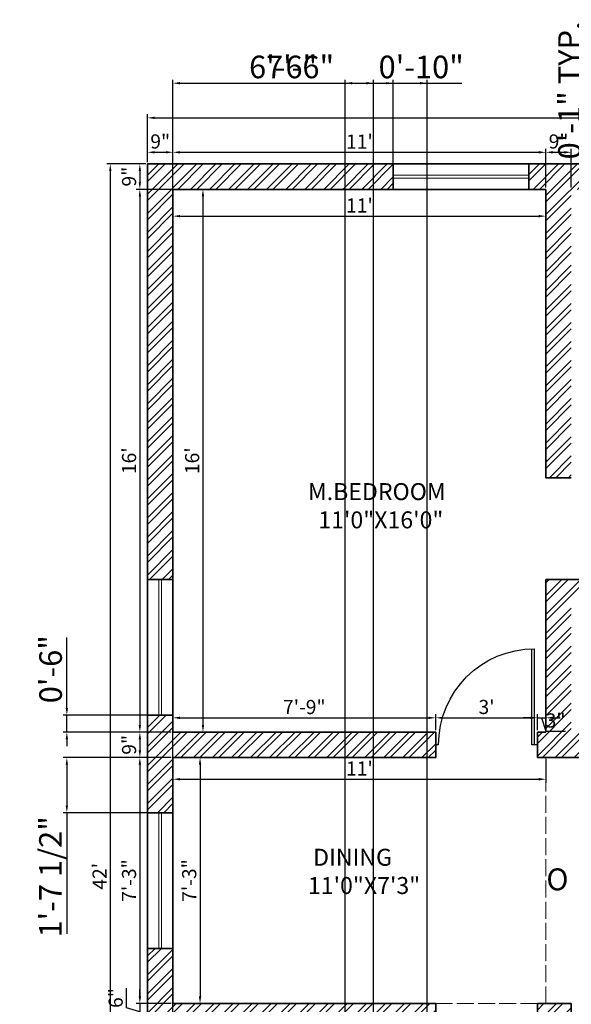
# Model space of a CAD drawing. Units: inches. Extents: x 3595 to 4516, y 2363 to 2965.
# Tile 3 of 12: x 3595 to 3790, y 2606 to 2954. Entities that reach past the tile are written whole.
import ezdxf

# ---------------------------------------------------------------- set-up
doc = ezdxf.new("R2010")
doc.units = ezdxf.units.IN
doc.linetypes.add('ACAD_ISO02W100', pattern=[15, 12, -3])
for name, color, linetype, lineweight in [('A-ANNO-DIMS', 2, 'Continuous', 18), ('A-ANNO-TEXT', 7, 'Continuous', 25), ('A-AREA-IDEN', 7, 'Continuous', 18), ('A-DOOR', 4, 'Continuous', 25), ('A-GLAZ', 4, 'Continuous', 18), ('A-WALL', 7, 'Continuous', 35), ('A-WALL-OVHD', 7, 'ACAD_ISO02W100', 18)]:
    doc.layers.add(name, color=color, linetype=linetype, lineweight=lineweight)
doc.layers.add('A-WALL-PATT', color=251, linetype='Continuous', lineweight=13, true_color=0x636466)
doc.styles.get("Standard").update_dxf_attribs({"font": 'arial.ttf'})
doc.dimstyles.new('ISO-25', dxfattribs={"dimtxt": 8, "dimasz": 2.5, "dimexe": 1.25, "dimexo": 0.625, "dimtad": 1, "dimdec": 1, "dimlunit": 3, "dimtxsty": 'Standard', "dimcen": 2.5, "dimadec": 0, "dimazin": 0, "dimtfac": 1, "dimtdec": 1, "dimtmove": 0, "dimatfit": 3, "dimfxl": 1, "dimarcsym": 0})

# ---------------------------------------------------------------- blocks, each defined once
blk = doc.blocks.new('D1')
for p, q in [((1, 0), (1, 34)), ((2, 0), (2, 33.99)), ((0, 0), (2, 0)), ((35, 0), (36, 0))]:
    blk.add_line(p, q)
at = {"ltscale": 0.5}
blk.add_arc((1, 0), 34, 0, 90, dxfattribs=at)
blk = doc.blocks.new('*D32')
at = {"layer": 'A-ANNO-DIMS', "color": 0, "lineweight": -2, "transparency": 16777216}
for p, q in [((3648.89, 2893.42), (3648.89, 2883.31)), ((3780.89, 2893.42), (3780.89, 2883.31)), ((3651.39, 2884.56), (3778.39, 2884.56))]:
    blk.add_line(p, q, dxfattribs=at)
at = {"layer": 'A-ANNO-DIMS', "color": 0, "transparency": 16777216}
for points in [[(3651.39, 2884.97), (3651.39, 2884.14), (3648.89, 2884.56)], [(3778.39, 2884.97), (3778.39, 2884.14), (3780.89, 2884.56)]]:
    blk.add_solid(points, dxfattribs=at)
at = {"layer": 'Defpoints', "color": 0, "transparency": 16777216}
for p in [(3648.89, 2894.04), (3780.89, 2894.04), (3780.89, 2884.56)]:
    blk.add_point(p, dxfattribs=at)
at = {"layer": 'A-ANNO-DIMS', "color": 0, "transparency": 16777216, "insert": (3714.89, 2887.69), "char_height": 5, "attachment_point": 5}
blk.add_mtext("11'", dxfattribs=at)
blk = doc.blocks.new('*D33')
at = {"layer": 'A-ANNO-DIMS', "color": 0, "lineweight": -2, "transparency": 16777216}
for p, q in [((3649.52, 2894.04), (3660.77, 2894.04)), ((3659.52, 2891.54), (3659.52, 2704.54)), ((3649.52, 2702.04), (3660.77, 2702.04))]:
    blk.add_line(p, q, dxfattribs=at)
at = {"layer": 'A-ANNO-DIMS', "color": 0, "transparency": 16777216}
for points in [[(3659.1, 2891.54), (3659.94, 2891.54), (3659.52, 2894.04)], [(3659.1, 2704.54), (3659.94, 2704.54), (3659.52, 2702.04)]]:
    blk.add_solid(points, dxfattribs=at)
at = {"layer": 'Defpoints', "color": 0, "transparency": 16777216}
for p in [(3648.89, 2894.04), (3648.89, 2702.04), (3659.52, 2702.04)]:
    blk.add_point(p, dxfattribs=at)
at = {"layer": 'A-ANNO-DIMS', "color": 0, "transparency": 16777216, "insert": (3656.34, 2798.04), "char_height": 5, "attachment_point": 5, "rotation": 90}
blk.add_mtext("16'", dxfattribs=at)
blk = doc.blocks.new('*D34')
at = {"layer": 'A-ANNO-DIMS', "color": 0, "lineweight": -2, "transparency": 16777216}
for p, q in [((3648.89, 2702.67), (3648.89, 2708.35)), ((3651.39, 2707.1), (3739.39, 2707.1)), ((3741.89, 2702.67), (3741.89, 2708.35))]:
    blk.add_line(p, q, dxfattribs=at)
at = {"layer": 'A-ANNO-DIMS', "color": 0, "transparency": 16777216}
for points in [[(3651.39, 2707.51), (3651.39, 2706.68), (3648.89, 2707.1)], [(3739.39, 2707.51), (3739.39, 2706.68), (3741.89, 2707.1)]]:
    blk.add_solid(points, dxfattribs=at)
at = {"layer": 'Defpoints', "color": 0, "transparency": 16777216}
for p in [(3741.89, 2707.1), (3648.89, 2702.04), (3741.89, 2702.04)]:
    blk.add_point(p, dxfattribs=at)
at = {"layer": 'A-ANNO-DIMS', "color": 0, "transparency": 16777216, "insert": (3695.39, 2710.27), "char_height": 5, "attachment_point": 5}
blk.add_mtext('7\'-9"', dxfattribs=at)
blk = doc.blocks.new('*D35')
at = {"layer": 'A-ANNO-DIMS', "color": 0, "lineweight": -2, "transparency": 16777216}
for p, q in [((3741.89, 2702.67), (3741.89, 2708.35)), ((3744.39, 2707.1), (3775.39, 2707.1)), ((3777.89, 2702.67), (3777.89, 2708.35))]:
    blk.add_line(p, q, dxfattribs=at)
at = {"layer": 'A-ANNO-DIMS', "color": 0, "transparency": 16777216}
for points in [[(3744.39, 2707.51), (3744.39, 2706.68), (3741.89, 2707.1)], [(3775.39, 2707.51), (3775.39, 2706.68), (3777.89, 2707.1)]]:
    blk.add_solid(points, dxfattribs=at)
at = {"layer": 'Defpoints', "color": 0, "transparency": 16777216}
for p in [(3777.89, 2707.1), (3741.89, 2702.04), (3777.89, 2702.04)]:
    blk.add_point(p, dxfattribs=at)
at = {"layer": 'A-ANNO-DIMS', "color": 0, "transparency": 16777216, "insert": (3759.89, 2710.28), "char_height": 5, "attachment_point": 5}
blk.add_mtext("3'", dxfattribs=at)
blk = doc.blocks.new('*D36')
at = {"layer": 'A-ANNO-DIMS', "color": 0, "lineweight": -2, "transparency": 16777216}
for p, q in [((3775.39, 2707.1), (3772.89, 2707.1)), ((3777.89, 2702.67), (3777.89, 2708.35)), ((3777.89, 2707.1), (3780.89, 2707.1)), ((3777.89, 2707.1), (3780.89, 2707.1)), ((3779.39, 2707.1), (3780.82, 2702.35)), ((3780.89, 2706.47), (3780.89, 2705.85)), ((3783.39, 2707.1), (3785.89, 2707.1)), ((3780.82, 2702.35), (3787.81, 2702.35))]:
    blk.add_line(p, q, dxfattribs=at)
at = {"layer": 'A-ANNO-DIMS', "color": 0, "transparency": 16777216}
for points in [[(3775.39, 2707.51), (3775.39, 2706.68), (3777.89, 2707.1)], [(3783.39, 2707.51), (3783.39, 2706.68), (3780.89, 2707.1)]]:
    blk.add_solid(points, dxfattribs=at)
at = {"layer": 'Defpoints', "color": 0, "transparency": 16777216}
for p in [(3780.89, 2707.1), (3780.89, 2707.1), (3777.89, 2702.04)]:
    blk.add_point(p, dxfattribs=at)
at = {"layer": 'A-ANNO-DIMS', "color": 0, "transparency": 16777216, "insert": (3784.31, 2705.53), "char_height": 5, "attachment_point": 5}
blk.add_mtext('3"', dxfattribs=at)
blk = doc.blocks.new('*D46')
at = {"layer": 'A-ANNO-DIMS', "color": 0, "lineweight": -2, "transparency": 16777216}
for p, q in [((3649.52, 2693.04), (3659.74, 2693.04)), ((3658.49, 2690.54), (3658.49, 2608.54)), ((3649.52, 2606.04), (3659.74, 2606.04))]:
    blk.add_line(p, q, dxfattribs=at)
at = {"layer": 'A-ANNO-DIMS', "color": 0, "transparency": 16777216}
for points in [[(3658.07, 2690.54), (3658.91, 2690.54), (3658.49, 2693.04)], [(3658.07, 2608.54), (3658.91, 2608.54), (3658.49, 2606.04)]]:
    blk.add_solid(points, dxfattribs=at)
at = {"layer": 'Defpoints', "color": 0, "transparency": 16777216}
for p in [(3648.89, 2693.04), (3648.89, 2606.04), (3658.49, 2606.04)]:
    blk.add_point(p, dxfattribs=at)
at = {"layer": 'A-ANNO-DIMS', "color": 0, "transparency": 16777216, "insert": (3655.31, 2649.54), "char_height": 5, "attachment_point": 5, "rotation": 90}
blk.add_mtext('7\'-3"', dxfattribs=at)
blk = doc.blocks.new('*D47')
at = {"layer": 'A-ANNO-DIMS', "color": 0, "lineweight": -2, "transparency": 16777216}
for p, q in [((3648.89, 2692.42), (3648.89, 2684.12)), ((3780.89, 2692.42), (3780.89, 2684.12)), ((3651.39, 2685.37), (3778.39, 2685.37))]:
    blk.add_line(p, q, dxfattribs=at)
at = {"layer": 'A-ANNO-DIMS', "color": 0, "transparency": 16777216}
for points in [[(3651.39, 2685.79), (3651.39, 2684.95), (3648.89, 2685.37)], [(3778.39, 2685.79), (3778.39, 2684.95), (3780.89, 2685.37)]]:
    blk.add_solid(points, dxfattribs=at)
at = {"layer": 'Defpoints', "color": 0, "transparency": 16777216}
for p in [(3648.89, 2693.04), (3780.89, 2693.04), (3780.89, 2685.37)]:
    blk.add_point(p, dxfattribs=at)
at = {"layer": 'A-ANNO-DIMS', "color": 0, "transparency": 16777216, "insert": (3714.89, 2688.5), "char_height": 5, "attachment_point": 5}
blk.add_mtext("11'", dxfattribs=at)
blk = doc.blocks.new('*D51')
at = {"layer": 'A-ANNO-DIMS', "color": 0, "lineweight": -2, "transparency": 16777216}
for p, q in [((3790.52, 2693.04), (3802.44, 2693.04)), ((3801.19, 2488.54), (3801.19, 2690.54)), ((3790.52, 2486.04), (3802.44, 2486.04))]:
    blk.add_line(p, q, dxfattribs=at)
at = {"layer": 'A-ANNO-DIMS', "color": 0, "transparency": 16777216}
for points in [[(3800.78, 2690.54), (3801.61, 2690.54), (3801.19, 2693.04)], [(3800.78, 2488.54), (3801.61, 2488.54), (3801.19, 2486.04)]]:
    blk.add_solid(points, dxfattribs=at)
at = {"layer": 'Defpoints', "color": 0, "transparency": 16777216}
for p in [(3789.89, 2693.04), (3801.19, 2693.04), (3789.89, 2486.04)]:
    blk.add_point(p, dxfattribs=at)
at = {"layer": 'A-ANNO-DIMS', "color": 0, "transparency": 16777216, "insert": (3798.01, 2589.54), "char_height": 5, "attachment_point": 5, "rotation": 90}
blk.add_mtext('17\'-3"', dxfattribs=at)
blk = doc.blocks.new('*D60')
at = {"layer": 'A-ANNO-DIMS', "color": 0, "lineweight": -2, "transparency": 16777216}
for p, q in [((3639.89, 2903.67), (3639.89, 2908.4)), ((3648.89, 2894.67), (3648.89, 2908.4)), ((3642.39, 2907.15), (3646.39, 2907.15))]:
    blk.add_line(p, q, dxfattribs=at)
at = {"layer": 'A-ANNO-DIMS', "color": 0, "transparency": 16777216}
for points in [[(3642.39, 2907.57), (3642.39, 2906.73), (3639.89, 2907.15)], [(3646.39, 2907.57), (3646.39, 2906.73), (3648.89, 2907.15)]]:
    blk.add_solid(points, dxfattribs=at)
at = {"layer": 'Defpoints', "color": 0, "transparency": 16777216}
for p in [(3648.89, 2907.15), (3639.89, 2903.04), (3648.89, 2894.04)]:
    blk.add_point(p, dxfattribs=at)
at = {"layer": 'A-ANNO-DIMS', "color": 0, "transparency": 16777216, "insert": (3644.39, 2910.33), "char_height": 5, "attachment_point": 5}
blk.add_mtext('9"', dxfattribs=at)
blk = doc.blocks.new('*D61')
at = {"layer": 'A-ANNO-DIMS', "color": 0, "lineweight": -2, "transparency": 16777216}
for p, q in [((3648.89, 2894.67), (3648.89, 2908.4)), ((3780.89, 2894.67), (3780.89, 2908.4)), ((3651.39, 2907.15), (3778.39, 2907.15))]:
    blk.add_line(p, q, dxfattribs=at)
at = {"layer": 'A-ANNO-DIMS', "color": 0, "transparency": 16777216}
for points in [[(3651.39, 2907.57), (3651.39, 2906.73), (3648.89, 2907.15)], [(3778.39, 2907.57), (3778.39, 2906.73), (3780.89, 2907.15)]]:
    blk.add_solid(points, dxfattribs=at)
at = {"layer": 'Defpoints', "color": 0, "transparency": 16777216}
for p in [(3780.89, 2907.15), (3648.89, 2894.04), (3780.89, 2894.04)]:
    blk.add_point(p, dxfattribs=at)
at = {"layer": 'A-ANNO-DIMS', "color": 0, "transparency": 16777216, "insert": (3714.89, 2910.29), "char_height": 5, "attachment_point": 5}
blk.add_mtext("11'", dxfattribs=at)
blk = doc.blocks.new('*D62')
at = {"layer": 'A-ANNO-DIMS', "color": 0, "lineweight": -2, "transparency": 16777216}
for p, q in [((3780.89, 2894.67), (3780.89, 2908.4)), ((3789.89, 2894.67), (3789.89, 2908.4)), ((3783.39, 2907.15), (3787.39, 2907.15))]:
    blk.add_line(p, q, dxfattribs=at)
at = {"layer": 'A-ANNO-DIMS', "color": 0, "transparency": 16777216}
for points in [[(3783.39, 2907.57), (3783.39, 2906.73), (3780.89, 2907.15)], [(3787.39, 2907.57), (3787.39, 2906.73), (3789.89, 2907.15)]]:
    blk.add_solid(points, dxfattribs=at)
at = {"layer": 'Defpoints', "color": 0, "transparency": 16777216}
for p in [(3789.89, 2907.15), (3780.89, 2894.04), (3789.89, 2894.04)]:
    blk.add_point(p, dxfattribs=at)
at = {"layer": 'A-ANNO-DIMS', "color": 0, "transparency": 16777216, "insert": (3785.39, 2910.33), "char_height": 5, "attachment_point": 5}
blk.add_mtext('9"', dxfattribs=at)
blk = doc.blocks.new('*D69')
at = {"layer": 'A-ANNO-DIMS', "color": 0, "lineweight": -2, "transparency": 16777216}
for p, q in [((3639.27, 2903.04), (3635.93, 2903.04)), ((3637.18, 2900.54), (3637.18, 2896.54)), ((3648.27, 2894.04), (3635.93, 2894.04))]:
    blk.add_line(p, q, dxfattribs=at)
at = {"layer": 'A-ANNO-DIMS', "color": 0, "transparency": 16777216}
for points in [[(3636.77, 2900.54), (3637.6, 2900.54), (3637.18, 2903.04)], [(3636.77, 2896.54), (3637.6, 2896.54), (3637.18, 2894.04)]]:
    blk.add_solid(points, dxfattribs=at)
at = {"layer": 'Defpoints', "color": 0, "transparency": 16777216}
for p in [(3639.89, 2903.04), (3637.18, 2894.04), (3648.89, 2894.04)]:
    blk.add_point(p, dxfattribs=at)
at = {"layer": 'A-ANNO-DIMS', "color": 0, "transparency": 16777216, "insert": (3634.01, 2898.54), "char_height": 5, "attachment_point": 5, "rotation": 90}
blk.add_mtext('9"', dxfattribs=at)
blk = doc.blocks.new('*D70')
at = {"layer": 'A-ANNO-DIMS', "color": 0, "lineweight": -2, "transparency": 16777216}
for p, q in [((3648.27, 2894.04), (3635.93, 2894.04)), ((3637.18, 2891.54), (3637.18, 2704.54)), ((3648.27, 2702.04), (3635.93, 2702.04))]:
    blk.add_line(p, q, dxfattribs=at)
at = {"layer": 'A-ANNO-DIMS', "color": 0, "transparency": 16777216}
for points in [[(3636.77, 2891.54), (3637.6, 2891.54), (3637.18, 2894.04)], [(3636.77, 2704.54), (3637.6, 2704.54), (3637.18, 2702.04)]]:
    blk.add_solid(points, dxfattribs=at)
at = {"layer": 'Defpoints', "color": 0, "transparency": 16777216}
for p in [(3648.89, 2894.04), (3637.18, 2702.04), (3648.89, 2702.04)]:
    blk.add_point(p, dxfattribs=at)
at = {"layer": 'A-ANNO-DIMS', "color": 0, "transparency": 16777216, "insert": (3634.01, 2798.04), "char_height": 5, "attachment_point": 5, "rotation": 90}
blk.add_mtext("16'", dxfattribs=at)
blk = doc.blocks.new('*D71')
at = {"layer": 'A-ANNO-DIMS', "color": 0, "lineweight": -2, "transparency": 16777216}
for p, q in [((3648.27, 2702.04), (3635.93, 2702.04)), ((3637.18, 2699.54), (3637.18, 2695.54)), ((3648.27, 2693.04), (3635.93, 2693.04))]:
    blk.add_line(p, q, dxfattribs=at)
at = {"layer": 'A-ANNO-DIMS', "color": 0, "transparency": 16777216}
for points in [[(3636.77, 2699.54), (3637.6, 2699.54), (3637.18, 2702.04)], [(3636.77, 2695.54), (3637.6, 2695.54), (3637.18, 2693.04)]]:
    blk.add_solid(points, dxfattribs=at)
at = {"layer": 'Defpoints', "color": 0, "transparency": 16777216}
for p in [(3648.89, 2702.04), (3637.18, 2693.04), (3648.89, 2693.04)]:
    blk.add_point(p, dxfattribs=at)
at = {"layer": 'A-ANNO-DIMS', "color": 0, "transparency": 16777216, "insert": (3634.01, 2697.54), "char_height": 5, "attachment_point": 5, "rotation": 90}
blk.add_mtext('9"', dxfattribs=at)
blk = doc.blocks.new('*D72')
at = {"layer": 'A-ANNO-DIMS', "color": 0, "lineweight": -2, "transparency": 16777216}
for p, q in [((3648.27, 2693.04), (3635.93, 2693.04)), ((3637.18, 2690.54), (3637.18, 2608.54)), ((3648.27, 2606.04), (3635.93, 2606.04))]:
    blk.add_line(p, q, dxfattribs=at)
at = {"layer": 'A-ANNO-DIMS', "color": 0, "transparency": 16777216}
for points in [[(3636.77, 2690.54), (3637.6, 2690.54), (3637.18, 2693.04)], [(3636.77, 2608.54), (3637.6, 2608.54), (3637.18, 2606.04)]]:
    blk.add_solid(points, dxfattribs=at)
at = {"layer": 'Defpoints', "color": 0, "transparency": 16777216}
for p in [(3648.89, 2693.04), (3637.18, 2606.04), (3648.89, 2606.04)]:
    blk.add_point(p, dxfattribs=at)
at = {"layer": 'A-ANNO-DIMS', "color": 0, "transparency": 16777216, "insert": (3634, 2649.54), "char_height": 5, "attachment_point": 5, "rotation": 90}
blk.add_mtext('7\'-3"', dxfattribs=at)
blk = doc.blocks.new('*D73')
at = {"layer": 'A-ANNO-DIMS', "color": 0, "lineweight": -2, "transparency": 16777216}
for p, q in [((3632.44, 2604.47), (3632.44, 2611.49)), ((3637.18, 2608.54), (3637.18, 2611.04)), ((3648.27, 2606.04), (3635.93, 2606.04)), ((3637.18, 2606.04), (3637.18, 2600.04)), ((3637.18, 2606.04), (3637.18, 2600.04)), ((3637.18, 2603.04), (3632.44, 2604.47)), ((3648.27, 2600.04), (3635.93, 2600.04)), ((3637.18, 2597.54), (3637.18, 2595.04))]:
    blk.add_line(p, q, dxfattribs=at)
at = {"layer": 'A-ANNO-DIMS', "color": 0, "transparency": 16777216}
for points in [[(3636.77, 2608.54), (3637.6, 2608.54), (3637.18, 2606.04)], [(3636.77, 2597.54), (3637.6, 2597.54), (3637.18, 2600.04)]]:
    blk.add_solid(points, dxfattribs=at)
at = {"layer": 'Defpoints', "color": 0, "transparency": 16777216}
for p in [(3648.89, 2606.04), (3637.18, 2600.04), (3648.89, 2600.04)]:
    blk.add_point(p, dxfattribs=at)
at = {"layer": 'A-ANNO-DIMS', "color": 0, "transparency": 16777216, "insert": (3629.27, 2607.98), "char_height": 5, "attachment_point": 5, "rotation": 90}
blk.add_mtext('6"', dxfattribs=at)
blk = doc.blocks.new('*D89')
at = {"layer": 'A-ANNO-DIMS', "color": 0, "lineweight": -2, "transparency": 16777216}
for p, q in [((3639.89, 2903.67), (3639.89, 2920.58)), ((3642.39, 2919.33), (3997.39, 2919.33)), ((3999.89, 2903.67), (3999.89, 2920.58))]:
    blk.add_line(p, q, dxfattribs=at)
at = {"layer": 'A-ANNO-DIMS', "color": 0, "transparency": 16777216}
for points in [[(3642.39, 2919.75), (3642.39, 2918.91), (3639.89, 2919.33)], [(3997.39, 2919.75), (3997.39, 2918.91), (3999.89, 2919.33)]]:
    blk.add_solid(points, dxfattribs=at)
at = {"layer": 'Defpoints', "color": 0, "transparency": 16777216}
for p in [(3999.89, 2919.33), (3639.89, 2903.04), (3999.89, 2903.04)]:
    blk.add_point(p, dxfattribs=at)
at = {"layer": 'A-ANNO-DIMS', "color": 0, "transparency": 16777216, "insert": (3819.89, 2922.51), "char_height": 5, "attachment_point": 5}
blk.add_mtext("30'", dxfattribs=at)
blk = doc.blocks.new('*D90')
at = {"layer": 'A-ANNO-DIMS', "color": 0, "lineweight": -2, "transparency": 16777216}
for p, q in [((3639.27, 2903.04), (3625.46, 2903.04)), ((3626.71, 2900.54), (3626.71, 2401.54)), ((3639.27, 2399.04), (3625.46, 2399.04))]:
    blk.add_line(p, q, dxfattribs=at)
at = {"layer": 'A-ANNO-DIMS', "color": 0, "transparency": 16777216}
for points in [[(3626.3, 2900.54), (3627.13, 2900.54), (3626.71, 2903.04)], [(3626.3, 2401.54), (3627.13, 2401.54), (3626.71, 2399.04)]]:
    blk.add_solid(points, dxfattribs=at)
at = {"layer": 'Defpoints', "color": 0, "transparency": 16777216}
for p in [(3639.89, 2903.04), (3626.71, 2399.04), (3639.89, 2399.04)]:
    blk.add_point(p, dxfattribs=at)
at = {"layer": 'A-ANNO-DIMS', "color": 0, "transparency": 16777216, "insert": (3623.58, 2651.04), "char_height": 5, "attachment_point": 5, "rotation": 90}
blk.add_mtext("42'", dxfattribs=at)
blk = doc.blocks.new('WIN-GLAZING-48IN')
for p, q in [((0, 1), (48, 1)), ((0, 0), (48, 0))]:
    blk.add_line(p, q)
blk = doc.blocks.new('*D108')
at = {"layer": 'A-ANNO-DIMS', "color": 0, "lineweight": -2, "transparency": 16777216}
for p, q in [((3794.99, 2901.54), (3794.99, 2954.06)), ((3799.77, 2899.04), (3793.74, 2899.04)), ((3799.77, 2898.04), (3793.74, 2898.04)), ((3794.99, 2898.04), (3794.99, 2899.04)), ((3794.99, 2895.54), (3794.99, 2893.04))]:
    blk.add_line(p, q, dxfattribs=at)
at = {"layer": 'A-ANNO-DIMS', "color": 0, "transparency": 16777216}
for points in [[(3794.58, 2901.54), (3795.41, 2901.54), (3794.99, 2899.04)], [(3794.58, 2895.54), (3795.41, 2895.54), (3794.99, 2898.04)]]:
    blk.add_solid(points, dxfattribs=at)
at = {"layer": 'Defpoints', "color": 0, "transparency": 16777216}
for p in [(3794.99, 2899.04), (3800.39, 2899.04), (3800.39, 2898.04)]:
    blk.add_point(p, dxfattribs=at)
at = {"layer": 'A-ANNO-DIMS', "color": 0, "transparency": 16777216, "insert": (3790.28, 2929.05), "char_height": 8, "attachment_point": 5, "rotation": 90}
blk.add_mtext('0\'-1" TYP.', dxfattribs=at)
blk = doc.blocks.new('*D147')
at = {"layer": 'A-ANNO-DIMS', "color": 0, "lineweight": -2, "transparency": 16777216}
for p, q in [((3648.89, 2894.67), (3648.89, 2932.84)), ((3726.89, 2894.67), (3726.89, 2932.84)), ((3651.39, 2931.59), (3724.39, 2931.59))]:
    blk.add_line(p, q, dxfattribs=at)
at = {"layer": 'A-ANNO-DIMS', "color": 0, "transparency": 16777216}
for points in [[(3651.39, 2932.01), (3651.39, 2931.18), (3648.89, 2931.59)], [(3724.39, 2932.01), (3724.39, 2931.18), (3726.89, 2931.59)]]:
    blk.add_solid(points, dxfattribs=at)
at = {"layer": 'Defpoints', "color": 0, "transparency": 16777216}
for p in [(3726.89, 2931.59), (3648.89, 2894.04), (3726.89, 2894.04)]:
    blk.add_point(p, dxfattribs=at)
at = {"layer": 'A-ANNO-DIMS', "color": 0, "transparency": 16777216, "insert": (3687.89, 2936.3), "char_height": 8, "attachment_point": 5}
blk.add_mtext('6\'-6"', dxfattribs=at)
blk = doc.blocks.new('*D150')
at = {"layer": 'A-ANNO-DIMS', "color": 0, "lineweight": -2, "transparency": 16777216}
for p, q in [((3611.34, 2710.54), (3611.34, 2735.56)), ((3648.27, 2708.04), (3610.09, 2708.04)), ((3611.34, 2702.04), (3611.34, 2708.04)), ((3648.27, 2702.04), (3610.09, 2702.04)), ((3611.34, 2699.54), (3611.34, 2697.04))]:
    blk.add_line(p, q, dxfattribs=at)
at = {"layer": 'A-ANNO-DIMS', "color": 0, "transparency": 16777216}
for points in [[(3610.93, 2710.54), (3611.76, 2710.54), (3611.34, 2708.04)], [(3610.93, 2699.54), (3611.76, 2699.54), (3611.34, 2702.04)]]:
    blk.add_solid(points, dxfattribs=at)
at = {"layer": 'Defpoints', "color": 0, "transparency": 16777216}
for p in [(3611.34, 2708.04), (3648.89, 2708.04), (3648.89, 2702.04)]:
    blk.add_point(p, dxfattribs=at)
at = {"layer": 'A-ANNO-DIMS', "color": 0, "transparency": 16777216, "insert": (3606.63, 2724.3), "char_height": 8, "attachment_point": 5, "rotation": 90}
blk.add_mtext('0\'-6"', dxfattribs=at)
blk = doc.blocks.new('*D151')
at = {"layer": 'A-ANNO-DIMS', "color": 0, "lineweight": -2, "transparency": 16777216}
for p, q in [((3648.27, 2693.04), (3610.09, 2693.04)), ((3611.34, 2690.54), (3611.34, 2676.04)), ((3648.27, 2673.54), (3610.09, 2673.54)), ((3611.34, 2673.54), (3611.34, 2630.64))]:
    blk.add_line(p, q, dxfattribs=at)
at = {"layer": 'A-ANNO-DIMS', "color": 0, "transparency": 16777216}
for points in [[(3610.93, 2690.54), (3611.76, 2690.54), (3611.34, 2693.04)], [(3610.93, 2676.04), (3611.76, 2676.04), (3611.34, 2673.54)]]:
    blk.add_solid(points, dxfattribs=at)
at = {"layer": 'Defpoints', "color": 0, "transparency": 16777216}
for p in [(3648.89, 2693.04), (3611.34, 2673.54), (3648.89, 2673.54)]:
    blk.add_point(p, dxfattribs=at)
at = {"layer": 'A-ANNO-DIMS', "color": 0, "transparency": 16777216, "insert": (3606.58, 2650.84), "char_height": 8, "attachment_point": 5, "rotation": 90}
blk.add_mtext('1\'-7 1/2"', dxfattribs=at)
blk = doc.blocks.new('*D156')
at = {"layer": 'A-ANNO-DIMS', "color": 0, "lineweight": -2, "transparency": 16777216}
for p, q in [((3648.89, 2486.67), (3648.89, 2932.84)), ((3738.89, 2486.67), (3738.89, 2932.84)), ((3651.39, 2931.59), (3736.39, 2931.59))]:
    blk.add_line(p, q, dxfattribs=at)
at = {"layer": 'A-ANNO-DIMS', "color": 0, "transparency": 16777216}
for points in [[(3651.39, 2932.01), (3651.39, 2931.18), (3648.89, 2931.59)], [(3736.39, 2932.01), (3736.39, 2931.18), (3738.89, 2931.59)]]:
    blk.add_solid(points, dxfattribs=at)
at = {"layer": 'Defpoints', "color": 0, "transparency": 16777216}
for p in [(3738.89, 2931.59), (3648.89, 2486.04), (3738.89, 2486.04)]:
    blk.add_point(p, dxfattribs=at)
at = {"layer": 'A-ANNO-DIMS', "color": 0, "transparency": 16777216, "insert": (3693.89, 2936.3), "char_height": 8, "attachment_point": 5}
blk.add_mtext('7\'-6"', dxfattribs=at)
blk = doc.blocks.new('*D159')
at = {"layer": 'A-ANNO-DIMS', "color": 0, "lineweight": -2, "transparency": 16777216}
for p, q in [((3709.89, 2405.67), (3709.89, 2932.84)), ((3719.89, 2405.67), (3719.89, 2932.84)), ((3712.39, 2931.59), (3717.39, 2931.59)), ((3719.89, 2931.59), (3751.12, 2931.59))]:
    blk.add_line(p, q, dxfattribs=at)
at = {"layer": 'A-ANNO-DIMS', "color": 0, "transparency": 16777216}
for points in [[(3712.39, 2932.01), (3712.39, 2931.18), (3709.89, 2931.59)], [(3717.39, 2932.01), (3717.39, 2931.18), (3719.89, 2931.59)]]:
    blk.add_solid(points, dxfattribs=at)
at = {"layer": 'Defpoints', "color": 0, "transparency": 16777216}
for p in [(3719.89, 2931.59), (3709.89, 2405.04), (3719.89, 2405.04)]:
    blk.add_point(p, dxfattribs=at)
at = {"layer": 'A-ANNO-DIMS', "color": 0, "transparency": 16777216, "insert": (3736.76, 2936.3), "char_height": 8, "attachment_point": 5}
blk.add_mtext('0\'-10"', dxfattribs=at)

msp = doc.modelspace()

# ---------------------------------------------------------------- hatches: boundary and pattern name
at = {"layer": 'A-WALL-PATT'}
h = msp.add_hatch(dxfattribs=at)
h.set_pattern_fill('ANSI32', color=256, scale=0.5)
h.paths.add_polyline_path([(3648.89, 2894.04), (3726.89, 2894.04), (3726.89, 2903.04), (3639.89, 2903.04), (3639.89, 2756.04), (3648.89, 2756.04)])
h.paths.add_polyline_path([(3800.39, 2903.04), (3774.89, 2903.04), (3774.89, 2894.04), (3780.89, 2894.04), (3780.89, 2792.04), (3789.89, 2792.04), (3789.89, 2894.04), (3800.39, 2894.04)])
h.paths.add_polyline_path([(3882.89, 2903.04), (3836.39, 2903.04), (3836.39, 2894.04), (3846.89, 2894.04), (3846.89, 2798.04), (3819.89, 2798.04), (3819.89, 2792.04), (3846.89, 2792.04), (3846.89, 2756.04), (3780.89, 2756.04), (3780.89, 2702.04), (3777.89, 2702.04), (3777.89, 2693.04), (3800.39, 2693.04), (3800.39, 2702.04), (3789.89, 2702.04), (3789.89, 2750.04), (3846.89, 2750.04), (3846.89, 2702.04), (3836.39, 2702.04), (3836.39, 2693.04), (3951.89, 2693.04), (3951.89, 2702.04), (3852.89, 2702.04), (3852.89, 2840.04), (3954.89, 2840.04), (3954.89, 2846.04), (3852.89, 2846.04), (3852.89, 2894.04), (3882.89, 2894.04)])
h.paths.add_polyline_path([(3999.89, 2903.04), (3918.89, 2903.04), (3918.89, 2894.04), (3948.89, 2894.04), (3948.89, 2876.04), (3954.89, 2876.04), (3954.89, 2894.04), (3990.89, 2894.04), (3990.89, 2795.04), (3999.89, 2795.04)])
h.paths.add_polyline_path([(3741.89, 2702.04), (3648.89, 2702.04), (3648.89, 2708.04), (3639.89, 2708.04), (3639.89, 2673.54), (3648.89, 2673.54), (3648.89, 2693.04), (3741.89, 2693.04)])
h.paths.add_polyline_path([(3648.89, 2600.04), (3741.89, 2600.04), (3741.89, 2606.04), (3648.89, 2606.04), (3648.89, 2625.54), (3639.89, 2625.54), (3639.89, 2561.04), (3648.89, 2561.04)])
h.paths.add_polyline_path([(3648.89, 2525.04), (3639.89, 2525.04), (3639.89, 2399.04), (3789.89, 2399.04), (3789.89, 2405.04), (3648.89, 2405.04), (3648.89, 2477.04), (3738.89, 2477.04), (3738.89, 2486.04), (3648.89, 2486.04)])
h.paths.add_polyline_path([(3789.89, 2606.04), (3777.89, 2606.04), (3777.89, 2600.04), (3780.89, 2600.04), (3780.89, 2486.04), (3774.89, 2486.04), (3774.89, 2477.04), (3831.89, 2477.04), (3831.89, 2486.04), (3789.89, 2486.04)])
h.paths.add_polyline_path([(3939.89, 2486.04), (3897.89, 2486.04), (3897.89, 2477.04), (3939.89, 2477.04)])
h.paths.add_polyline_path([(3999.89, 2511.54), (3990.89, 2511.54), (3990.89, 2486.04), (3987.89, 2486.04), (3987.89, 2477.04), (3999.89, 2477.04)])
h.paths.add_polyline_path([(3999.89, 2607.54), (3990.89, 2607.54), (3990.89, 2571.54), (3999.89, 2571.54)])
h.paths.add_polyline_path([(3999.89, 2747.04), (3990.89, 2747.04), (3990.89, 2702.04), (3987.89, 2702.04), (3987.89, 2693.04), (3990.89, 2693.04), (3990.89, 2667.54), (3999.89, 2667.54)])

# ---------------------------------------------------------------- linework, layer by layer
at = {"layer": 'A-WALL'}
for p, q in [((3726.89, 2894.04), (3726.89, 2903.04)), ((3774.89, 2894.04), (3774.89, 2903.04)), ((3648.89, 2894.04), (3780.89, 2894.04)), ((3648.89, 2702.04), (3648.89, 2894.04)), ((3780.89, 2792.04), (3780.89, 2894.04)), ((3780.89, 2792.04), (3789.89, 2792.04)), ((3639.89, 2756.04), (3648.89, 2756.04)), ((3780.89, 2756.04), (3846.89, 2756.04)), ((3780.89, 2702.04), (3780.89, 2756.04)), ((3639.89, 2708.04), (3648.89, 2708.04)), ((3648.89, 2702.04), (3741.89, 2702.04)), ((3741.89, 2693.04), (3741.89, 2702.04)), ((3777.89, 2693.04), (3777.89, 2702.04)), ((3777.89, 2702.04), (3780.89, 2702.04)), ((3648.89, 2693.04), (3741.89, 2693.04)), ((3648.89, 2606.04), (3648.89, 2693.04)), ((3777.89, 2693.04), (3800.39, 2693.04)), ((3639.89, 2673.54), (3648.89, 2673.54)), ((3639.89, 2625.54), (3648.89, 2625.54)), ((3648.89, 2606.04), (3741.89, 2606.04)), ((3741.89, 2606.04), (3741.89, 2600.04)), ((3777.89, 2606.04), (3777.89, 2600.04)), ((3777.89, 2606.04), (3789.89, 2606.04)), ((3789.89, 2486.04), (3789.89, 2606.04))]:
    msp.add_line(p, q, dxfattribs=at)
msp.add_lwpolyline([(3789.89, 2399.04), (3639.89, 2399.04), (3639.89, 2903.04), (3999.89, 2903.04), (3999.89, 2477.04)], dxfattribs=at)
at = {"layer": 'A-WALL-OVHD', "ltscale": 0.5}
for p, q in [((3780.89, 2606.04), (3780.89, 2693.04)), ((3741.89, 2606.04), (3777.89, 2606.04))]:
    msp.add_line(p, q, dxfattribs=at)

# ---------------------------------------------------------------- block references
at = {"layer": 'A-DOOR', "xscale": -1}
msp.add_blockref('D1', (3777.89, 2697.54), dxfattribs=at)
at = {"layer": 'A-GLAZ'}
msp.add_blockref('WIN-GLAZING-48IN', (3726.89, 2898.04), dxfattribs=at)
at = {"layer": 'A-GLAZ', "rotation": 269.9999999999989}
for p in [(3643.89, 2756.04), (3643.89, 2673.54)]:
    msp.add_blockref('WIN-GLAZING-48IN', p, dxfattribs=at)

# ---------------------------------------------------------------- texts
at = {"layer": 'A-ANNO-TEXT'}
msp.add_text('O', height=7.75, dxfattribs=at).set_placement((3781.06, 2646.07))
at = {"layer": 'A-AREA-IDEN', "char_height": 6, "attachment_point": 1}
for s, insert in [('{\\fTimes New Roman|b0|i0|c0|p18;M.BEDROOM\\P  11\'0"X16\'0"}', (3696.68, 2790.12)), ('{\\fTimes New Roman|b0|i0|c0|p18; DINING\\P11\'0"X7\'3"}', (3696.68, 2660.77))]:
    msp.add_mtext_dynamic_manual_height_columns(s, width=67.3508, gutter_width=12.5, heights=[0], dxfattribs=dict(at, insert=insert))

# ---------------------------------------------------------------- dimensions: what is measured, and where the dimension line sits
at = {"layer": 'A-ANNO-DIMS'}
dim = msp.add_linear_dim(base=(3794.99, 2899.04), p1=(3800.39, 2898.04), p2=(3800.39, 2899.04), angle=90, text='<> TYP.', dimstyle='ISO-25', override={"dimdec": 1, "dimlfac": 1, "dimrnd": 0, "dimzin": 1, "dimdsep": 46, "dimlunit": 4, "dimfrac": 2}, dxfattribs=at)
dim.commit()
dim.dimension.update_dxf_attribs({"geometry": '*D108', "text_midpoint": (3790.28, 2929.05)})
for base, p1, p2, override, picture, middle in [((3726.89, 2931.59), (3648.89, 2894.04), (3726.89, 2894.04), {"dimdec": 1, "dimlfac": 1, "dimrnd": 0, "dimzin": 1, "dimdsep": 46, "dimlunit": 4, "dimfrac": 2}, '*D147', (3687.89, 2936.3)), ((3738.89, 2931.59), (3648.89, 2486.04), (3738.89, 2486.04), {"dimdec": 1, "dimlfac": 1, "dimrnd": 0, "dimzin": 1, "dimdsep": 46, "dimlunit": 4, "dimfrac": 2}, '*D156', (3693.89, 2936.3)), ((3719.89, 2931.59), (3709.89, 2405.04), (3719.89, 2405.04), {"dimdec": 1, "dimlfac": 1, "dimrnd": 0, "dimzin": 1, "dimdsep": 46, "dimlunit": 4, "dimfrac": 2}, '*D159', (3736.76, 2936.3)), ((3999.89, 2919.33), (3639.89, 2903.04), (3999.89, 2903.04), {"dimtxt": 5, "dimclrd": 0, "dimclre": 0, "dimclrt": 0}, '*D89', (3819.89, 2922.51)), ((3648.89, 2907.15), (3639.89, 2903.04), (3648.89, 2894.04), {"dimtxt": 5, "dimclrd": 0, "dimclre": 0, "dimclrt": 0}, '*D60', (3644.39, 2910.33)), ((3780.89, 2907.15), (3648.89, 2894.04), (3780.89, 2894.04), {"dimtxt": 5, "dimclrd": 0, "dimclre": 0, "dimclrt": 0, "dimtmove": 1}, '*D61', (3714.89, 2910.29)), ((3789.89, 2907.15), (3780.89, 2894.04), (3789.89, 2894.04), {"dimtxt": 5, "dimclrd": 0, "dimclre": 0, "dimclrt": 0, "dimtmove": 1}, '*D62', (3785.39, 2910.33)), ((3780.89, 2884.56), (3648.89, 2894.04), (3780.89, 2894.04), {"dimtxt": 5, "dimclrd": 0, "dimclre": 0, "dimclrt": 0}, '*D32', (3714.89, 2887.69)), ((3741.89, 2707.1), (3648.89, 2702.04), (3741.89, 2702.04), {"dimtxt": 5, "dimclrd": 0, "dimclre": 0, "dimclrt": 0}, '*D34', (3695.39, 2710.27)), ((3777.89, 2707.1), (3741.89, 2702.04), (3777.89, 2702.04), {"dimtxt": 5, "dimclrd": 0, "dimclre": 0, "dimclrt": 0, "dimtmove": 1}, '*D35', (3759.89, 2710.28)), ((3780.89, 2707.1), (3777.89, 2702.04), (3780.89, 2707.1), {"dimtxt": 5, "dimclrd": 0, "dimclre": 0, "dimclrt": 0, "dimtmove": 1}, '*D36', (3781.44, 2705.53)), ((3780.89, 2685.37), (3648.89, 2693.04), (3780.89, 2693.04), {"dimtxt": 5, "dimclrd": 0, "dimclre": 0, "dimclrt": 0}, '*D47', (3714.89, 2688.5))]:
    dim = msp.add_linear_dim(base=base, p1=p1, p2=p2, dimstyle='ISO-25', override=override, dxfattribs=at)
    dim.commit()
    dim.dimension.update_dxf_attribs({"geometry": picture, "text_midpoint": middle})
for base, p1, p2, override, picture, middle in [((3626.71, 2399.04), (3639.89, 2903.04), (3639.89, 2399.04), {"dimtxt": 5, "dimclrd": 0, "dimclre": 0, "dimclrt": 0}, '*D90', (3623.58, 2651.04)), ((3637.18, 2894.04), (3639.89, 2903.04), (3648.89, 2894.04), {"dimtxt": 5, "dimclrd": 0, "dimclre": 0, "dimclrt": 0}, '*D69', (3634.01, 2898.54)), ((3637.18, 2702.04), (3648.89, 2894.04), (3648.89, 2702.04), {"dimtxt": 5, "dimclrd": 0, "dimclre": 0, "dimclrt": 0, "dimtmove": 1}, '*D70', (3634.01, 2798.04)), ((3659.52, 2702.04), (3648.89, 2894.04), (3648.89, 2702.04), {"dimtxt": 5, "dimclrd": 0, "dimclre": 0, "dimclrt": 0}, '*D33', (3656.34, 2798.04)), ((3611.34, 2708.04), (3648.89, 2702.04), (3648.89, 2708.04), {"dimdec": 1, "dimlfac": 1, "dimrnd": 0, "dimzin": 1, "dimdsep": 46, "dimlunit": 4, "dimfrac": 2}, '*D150', (3606.63, 2724.3)), ((3637.18, 2693.04), (3648.89, 2702.04), (3648.89, 2693.04), {"dimtxt": 5, "dimclrd": 0, "dimclre": 0, "dimclrt": 0, "dimtmove": 1}, '*D71', (3634.01, 2697.54)), ((3611.34, 2673.54), (3648.89, 2693.04), (3648.89, 2673.54), {"dimdec": 1, "dimlfac": 1, "dimrnd": 0, "dimzin": 1, "dimdsep": 46, "dimlunit": 4, "dimfrac": 2}, '*D151', (3606.58, 2650.84)), ((3637.18, 2606.04), (3648.89, 2693.04), (3648.89, 2606.04), {"dimtxt": 5, "dimclrd": 0, "dimclre": 0, "dimclrt": 0, "dimtmove": 1}, '*D72', (3634, 2649.54)), ((3658.49, 2606.04), (3648.89, 2693.04), (3648.89, 2606.04), {"dimtxt": 5, "dimclrd": 0, "dimclre": 0, "dimclrt": 0}, '*D46', (3655.31, 2649.54)), ((3801.19, 2693.04), (3789.89, 2486.04), (3789.89, 2693.04), {"dimtxt": 5, "dimclrd": 0, "dimclre": 0, "dimclrt": 0}, '*D51', (3798.01, 2589.54)), ((3637.18, 2600.04), (3648.89, 2606.04), (3648.89, 2600.04), {"dimtxt": 5, "dimclrd": 0, "dimclre": 0, "dimclrt": 0, "dimtmove": 1}, '*D73', (3629.27, 2605.09))]:
    dim = msp.add_linear_dim(base=base, p1=p1, p2=p2, angle=90, dimstyle='ISO-25', override=override, dxfattribs=at)
    dim.commit()
    dim.dimension.update_dxf_attribs({"geometry": picture, "text_midpoint": middle})

doc.saveas('drawing.dxf')
